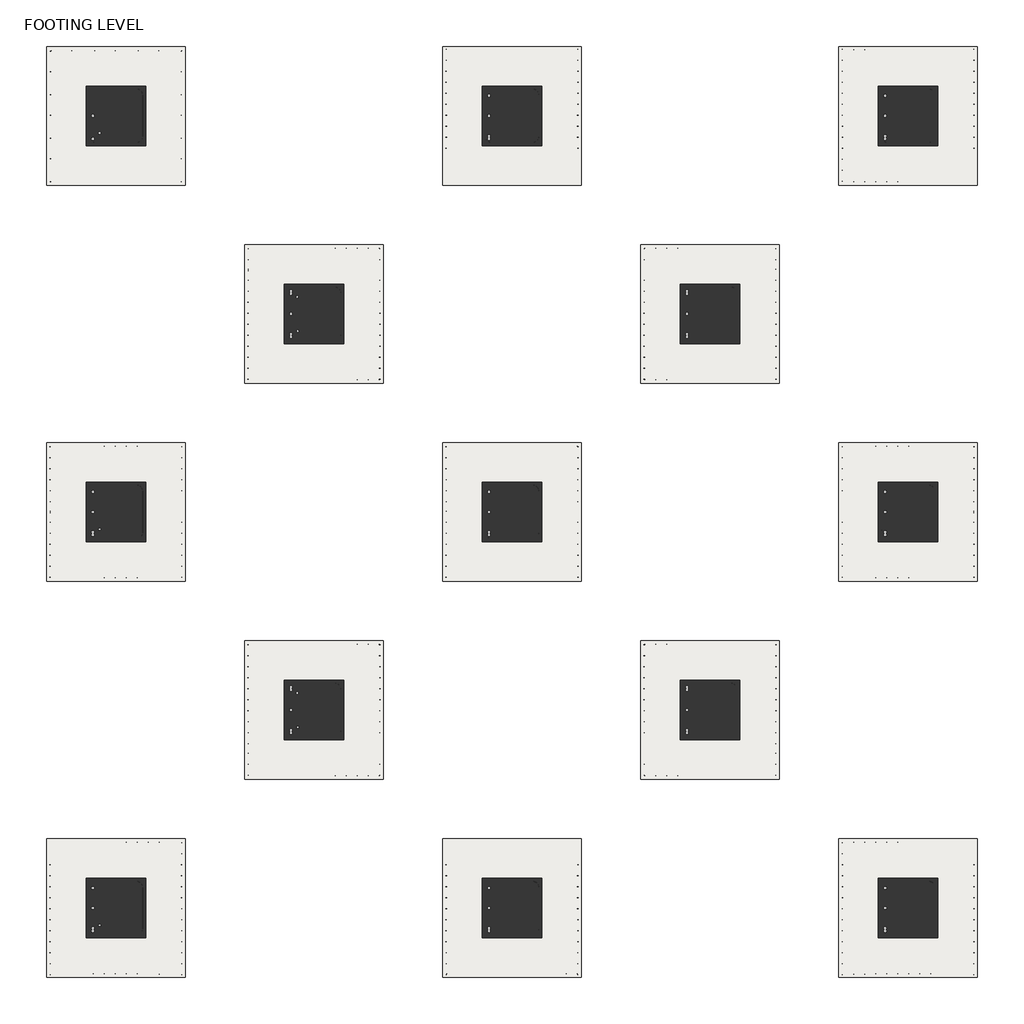
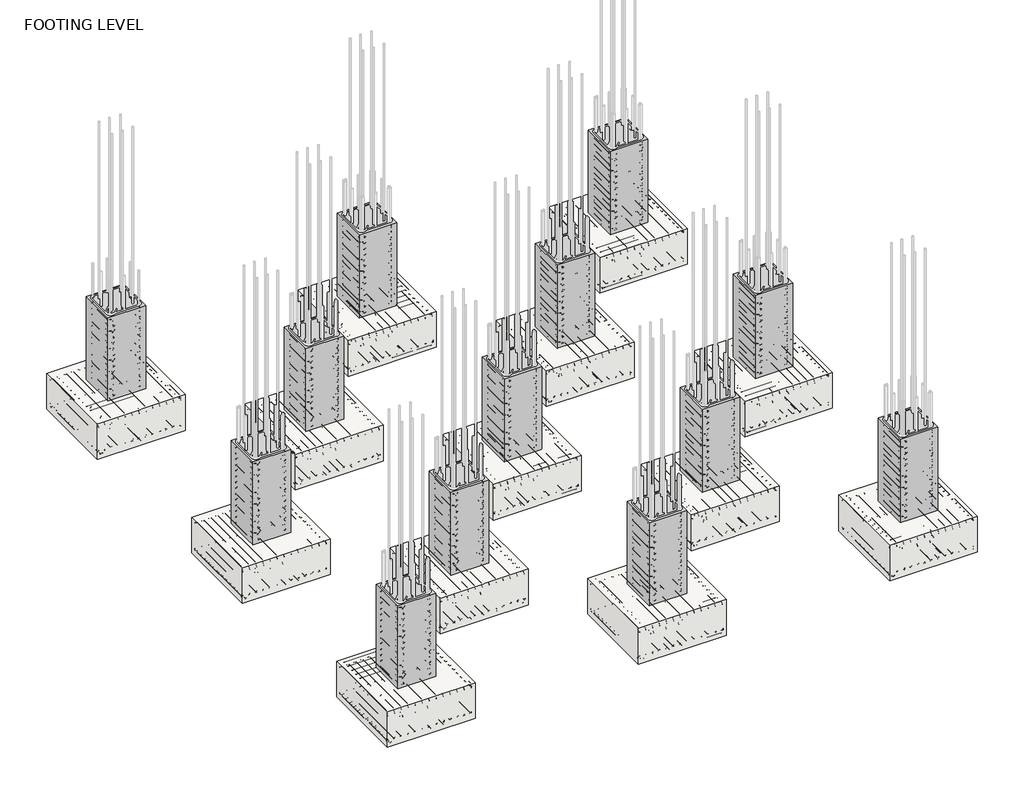
# One storey, part 1 of 10: 13 columns, 13 slabs.
"""IFC4 building model written with IfcOpenShell, lengths in millimetres."""

from ifc_helpers import new_model, si_unit, frame, origin, place, context, project, spatial, polyline, outline, extrude, transform, mapped, element, save
from components import m_footing_rectangular_1800_x_1200_x_450mm_ec84a8aa

model = new_model("IFC4")

# Units and contexts
model_context = context("Model", 3, world=origin())
ifc_project = project(units=[si_unit("LENGTHUNIT", "METRE", prefix="MILLI")], contexts=[model_context])

# Site, building, storey
site = spatial("IfcSite", under=ifc_project)
building = spatial("IfcBuilding", under=site)
storey = spatial("IfcBuildingStorey", under=building, Name="FOOTING LEVEL", Elevation=-2133.6)

# Columns
placement = place(None, origin())
element("IfcColumn", 1, ObjectType="M_Concrete-Rectangular-Column : 3'X3'", at=placement, inside=storey, context=model_context, shape_type="SweptSolid", body=[
    extrude(outline(polyline([(-12383.8269037, 12391.5829396), (-12383.8269037, 11477.1829396), (-13298.2269037, 11477.1829396), (-13298.2269037, 12391.5829396), (-12383.8269037, 12391.5829396)])), frame((0.0, 0.0, -2133.6), z_axis=(0.0, 0.0, 1.0), x_axis=(1.0, 0.0, 0.0)), (0.0, 0.0, 1.0), 2133.6),
])
element("IfcColumn", 2, ObjectType="M_Concrete-Rectangular-Column : 3'X3'", at=placement, inside=storey, context=model_context, shape_type="SweptSolid", body=[
    extrude(outline(polyline([(-12383.8269037, 6295.5829396), (-12383.8269037, 5381.1829396), (-13298.2269037, 5381.1829396), (-13298.2269037, 6295.5829396), (-12383.8269037, 6295.5829396)])), frame((0.0, 0.0, -2133.6), z_axis=(0.0, 0.0, 1.0), x_axis=(1.0, 0.0, 0.0)), (0.0, 0.0, 1.0), 2133.6),
])
element("IfcColumn", 3, ObjectType="M_Concrete-Rectangular-Column : 3'X3'", at=placement, inside=storey, context=model_context, shape_type="SweptSolid", body=[
    extrude(outline(polyline([(-12383.8269037, 199.5829396), (-12383.8269037, -714.8170604), (-13298.2269037, -714.8170604), (-13298.2269037, 199.5829396), (-12383.8269037, 199.5829396)])), frame((0.0, 0.0, -2133.6), z_axis=(0.0, 0.0, 1.0), x_axis=(1.0, 0.0, 0.0)), (0.0, 0.0, 1.0), 2133.6),
])
element("IfcColumn", 4, ObjectType="M_Concrete-Rectangular-Column : 3'X3'", at=placement, inside=storey, context=model_context, shape_type="SweptSolid", body=[
    extrude(outline(polyline([(-9335.8269037, 9343.5829396), (-9335.8269037, 8429.1829396), (-10250.2269037, 8429.1829396), (-10250.2269037, 9343.5829396), (-9335.8269037, 9343.5829396)])), frame((0.0, 0.0, -2133.6), z_axis=(0.0, 0.0, 1.0), x_axis=(1.0, 0.0, 0.0)), (0.0, 0.0, 1.0), 2133.6),
])
element("IfcColumn", 5, ObjectType="M_Concrete-Rectangular-Column : 3'X3'", at=placement, inside=storey, context=model_context, shape_type="SweptSolid", body=[
    extrude(outline(polyline([(-9335.8269037, 3247.5829396), (-9335.8269037, 2333.1829396), (-10250.2269037, 2333.1829396), (-10250.2269037, 3247.5829396), (-9335.8269037, 3247.5829396)])), frame((0.0, 0.0, -2133.6), z_axis=(0.0, 0.0, 1.0), x_axis=(1.0, 0.0, 0.0)), (0.0, 0.0, 1.0), 2133.6),
])
element("IfcColumn", 6, ObjectType="M_Concrete-Rectangular-Column : 3'X3'", at=placement, inside=storey, context=model_context, shape_type="SweptSolid", body=[
    extrude(outline(polyline([(-6287.8269037, 12391.5829396), (-6287.8269037, 11477.1829396), (-7202.2269037, 11477.1829396), (-7202.2269037, 12391.5829396), (-6287.8269037, 12391.5829396)])), frame((0.0, 0.0, -2133.6), z_axis=(0.0, 0.0, 1.0), x_axis=(1.0, 0.0, 0.0)), (0.0, 0.0, 1.0), 2133.6),
])
element("IfcColumn", 7, ObjectType="M_Concrete-Rectangular-Column : 3'X3'", at=placement, inside=storey, context=model_context, shape_type="SweptSolid", body=[
    extrude(outline(polyline([(-6287.8269037, 6295.5829396), (-6287.8269037, 5381.1829396), (-7202.2269037, 5381.1829396), (-7202.2269037, 6295.5829396), (-6287.8269037, 6295.5829396)])), frame((0.0, 0.0, -2133.6), z_axis=(0.0, 0.0, 1.0), x_axis=(1.0, 0.0, 0.0)), (0.0, 0.0, 1.0), 2133.6),
])
element("IfcColumn", 8, ObjectType="M_Concrete-Rectangular-Column : 3'X3'", at=placement, inside=storey, context=model_context, shape_type="SweptSolid", body=[
    extrude(outline(polyline([(-6287.8269037, 199.5829396), (-6287.8269037, -714.8170604), (-7202.2269037, -714.8170604), (-7202.2269037, 199.5829396), (-6287.8269037, 199.5829396)])), frame((0.0, 0.0, -2133.6), z_axis=(0.0, 0.0, 1.0), x_axis=(1.0, 0.0, 0.0)), (0.0, 0.0, 1.0), 2133.6),
])
element("IfcColumn", 9, ObjectType="M_Concrete-Rectangular-Column : 3'X3'", at=placement, inside=storey, context=model_context, shape_type="SweptSolid", body=[
    extrude(outline(polyline([(-3239.8269037, 9343.5829396), (-3239.8269037, 8429.1829396), (-4154.2269037, 8429.1829396), (-4154.2269037, 9343.5829396), (-3239.8269037, 9343.5829396)])), frame((0.0, 0.0, -2133.6), z_axis=(0.0, 0.0, 1.0), x_axis=(1.0, 0.0, 0.0)), (0.0, 0.0, 1.0), 2133.6),
])
element("IfcColumn", 10, ObjectType="M_Concrete-Rectangular-Column : 3'X3'", at=placement, inside=storey, context=model_context, shape_type="SweptSolid", body=[
    extrude(outline(polyline([(-3239.8269037, 3247.5829396), (-3239.8269037, 2333.1829396), (-4154.2269037, 2333.1829396), (-4154.2269037, 3247.5829396), (-3239.8269037, 3247.5829396)])), frame((0.0, 0.0, -2133.6), z_axis=(0.0, 0.0, 1.0), x_axis=(1.0, 0.0, 0.0)), (0.0, 0.0, 1.0), 2133.6),
])
element("IfcColumn", 11, ObjectType="M_Concrete-Rectangular-Column : 3'X3'", at=placement, inside=storey, context=model_context, shape_type="SweptSolid", body=[
    extrude(outline(polyline([(-191.8269037, 12391.5829396), (-191.8269037, 11477.1829396), (-1106.2269037, 11477.1829396), (-1106.2269037, 12391.5829396), (-191.8269037, 12391.5829396)])), frame((0.0, 0.0, -2133.6), z_axis=(0.0, 0.0, 1.0), x_axis=(1.0, 0.0, 0.0)), (0.0, 0.0, 1.0), 2133.6),
])
element("IfcColumn", 12, ObjectType="M_Concrete-Rectangular-Column : 3'X3'", at=placement, inside=storey, context=model_context, shape_type="SweptSolid", body=[
    extrude(outline(polyline([(-191.8269037, 6295.5829396), (-191.8269037, 5381.1829396), (-1106.2269037, 5381.1829396), (-1106.2269037, 6295.5829396), (-191.8269037, 6295.5829396)])), frame((0.0, 0.0, -2133.6), z_axis=(0.0, 0.0, 1.0), x_axis=(1.0, 0.0, 0.0)), (0.0, 0.0, 1.0), 2133.6),
])
element("IfcColumn", 13, ObjectType="M_Concrete-Rectangular-Column : 3'X3'", at=placement, inside=storey, context=model_context, shape_type="SweptSolid", body=[
    extrude(outline(polyline([(-191.8269037, 199.5829396), (-191.8269037, -714.8170604), (-1106.2269037, -714.8170604), (-1106.2269037, 199.5829396), (-191.8269037, 199.5829396)])), frame((0.0, 0.0, -2133.6), z_axis=(0.0, 0.0, 1.0), x_axis=(1.0, 0.0, 0.0)), (0.0, 0.0, 1.0), 2133.6),
])

# Slabs
m_footing_rectangular_1800_x_1200_x_450mm_shape = m_footing_rectangular_1800_x_1200_x_450mm_ec84a8aa(model_context)
element("IfcSlab", 14, ObjectType="M_Footing-Rectangular : 1800 x 1200 x 450mm", at=placement, inside=storey, context=model_context, shape_type="MappedRepresentation", body=[
    mapped(m_footing_rectangular_1800_x_1200_x_450mm_shape, transform((-12841.0269037, 11934.3829396, -2133.6), x_axis=(1.0, 0.0, 0.0), y_axis=(0.0, 1.0, 0.0), z_axis=(0.0, 0.0, 1.0))),
])
element("IfcSlab", 15, ObjectType="M_Footing-Rectangular : 1800 x 1200 x 450mm", at=placement, inside=storey, context=model_context, shape_type="MappedRepresentation", body=[
    mapped(m_footing_rectangular_1800_x_1200_x_450mm_shape, transform((-12841.0269037, 5838.3829396, -2133.6), x_axis=(1.0, 0.0, 0.0), y_axis=(0.0, 1.0, 0.0), z_axis=(0.0, 0.0, 1.0))),
])
element("IfcSlab", 16, ObjectType="M_Footing-Rectangular : 1800 x 1200 x 450mm", at=placement, inside=storey, context=model_context, shape_type="MappedRepresentation", body=[
    mapped(m_footing_rectangular_1800_x_1200_x_450mm_shape, transform((-12841.0269037, -257.6170604, -2133.6), x_axis=(1.0, 0.0, 0.0), y_axis=(0.0, 1.0, 0.0), z_axis=(0.0, 0.0, 1.0))),
])
element("IfcSlab", 17, ObjectType="M_Footing-Rectangular : 1800 x 1200 x 450mm", at=placement, inside=storey, context=model_context, shape_type="MappedRepresentation", body=[
    mapped(m_footing_rectangular_1800_x_1200_x_450mm_shape, transform((-9793.0269037, 8886.3829396, -2133.6), x_axis=(1.0, 0.0, 0.0), y_axis=(0.0, 1.0, 0.0), z_axis=(0.0, 0.0, 1.0))),
])
element("IfcSlab", 18, ObjectType="M_Footing-Rectangular : 1800 x 1200 x 450mm", at=placement, inside=storey, context=model_context, shape_type="MappedRepresentation", body=[
    mapped(m_footing_rectangular_1800_x_1200_x_450mm_shape, transform((-9793.0269037, 2790.3829396, -2133.6), x_axis=(1.0, 0.0, 0.0), y_axis=(0.0, 1.0, 0.0), z_axis=(0.0, 0.0, 1.0))),
])
element("IfcSlab", 19, ObjectType="M_Footing-Rectangular : 1800 x 1200 x 450mm", at=placement, inside=storey, context=model_context, shape_type="MappedRepresentation", body=[
    mapped(m_footing_rectangular_1800_x_1200_x_450mm_shape, transform((-6745.0269037, 11934.3829396, -2133.6), x_axis=(1.0, 0.0, 0.0), y_axis=(0.0, 1.0, 0.0), z_axis=(0.0, 0.0, 1.0))),
])
element("IfcSlab", 20, ObjectType="M_Footing-Rectangular : 1800 x 1200 x 450mm", at=placement, inside=storey, context=model_context, shape_type="MappedRepresentation", body=[
    mapped(m_footing_rectangular_1800_x_1200_x_450mm_shape, transform((-6745.0269037, 5838.3829396, -2133.6), x_axis=(1.0, 0.0, 0.0), y_axis=(0.0, 1.0, 0.0), z_axis=(0.0, 0.0, 1.0))),
])
element("IfcSlab", 21, ObjectType="M_Footing-Rectangular : 1800 x 1200 x 450mm", at=placement, inside=storey, context=model_context, shape_type="MappedRepresentation", body=[
    mapped(m_footing_rectangular_1800_x_1200_x_450mm_shape, transform((-6745.0269037, -257.6170604, -2133.6), x_axis=(1.0, 0.0, 0.0), y_axis=(0.0, 1.0, 0.0), z_axis=(0.0, 0.0, 1.0))),
])
element("IfcSlab", 22, ObjectType="M_Footing-Rectangular : 1800 x 1200 x 450mm", at=placement, inside=storey, context=model_context, shape_type="MappedRepresentation", body=[
    mapped(m_footing_rectangular_1800_x_1200_x_450mm_shape, transform((-3697.0269037, 8886.3829396, -2133.6), x_axis=(1.0, 0.0, 0.0), y_axis=(0.0, 1.0, 0.0), z_axis=(0.0, 0.0, 1.0))),
])
element("IfcSlab", 23, ObjectType="M_Footing-Rectangular : 1800 x 1200 x 450mm", at=placement, inside=storey, context=model_context, shape_type="MappedRepresentation", body=[
    mapped(m_footing_rectangular_1800_x_1200_x_450mm_shape, transform((-3697.0269037, 2790.3829396, -2133.6), x_axis=(1.0, 0.0, 0.0), y_axis=(0.0, 1.0, 0.0), z_axis=(0.0, 0.0, 1.0))),
])
element("IfcSlab", 24, ObjectType="M_Footing-Rectangular : 1800 x 1200 x 450mm", at=placement, inside=storey, context=model_context, shape_type="MappedRepresentation", body=[
    mapped(m_footing_rectangular_1800_x_1200_x_450mm_shape, transform((-649.0269037, 11934.3829396, -2133.6), x_axis=(1.0, 0.0, 0.0), y_axis=(0.0, 1.0, 0.0), z_axis=(0.0, 0.0, 1.0))),
])
element("IfcSlab", 25, ObjectType="M_Footing-Rectangular : 1800 x 1200 x 450mm", at=placement, inside=storey, context=model_context, shape_type="MappedRepresentation", body=[
    mapped(m_footing_rectangular_1800_x_1200_x_450mm_shape, transform((-649.0269037, 5838.3829396, -2133.6), x_axis=(1.0, 0.0, 0.0), y_axis=(0.0, 1.0, 0.0), z_axis=(0.0, 0.0, 1.0))),
])
element("IfcSlab", 26, ObjectType="M_Footing-Rectangular : 1800 x 1200 x 450mm", at=placement, inside=storey, context=model_context, shape_type="MappedRepresentation", body=[
    mapped(m_footing_rectangular_1800_x_1200_x_450mm_shape, transform((-649.0269037, -257.6170604, -2133.6), x_axis=(1.0, 0.0, 0.0), y_axis=(0.0, 1.0, 0.0), z_axis=(0.0, 0.0, 1.0))),
])

save(model, "model.ifc")

# Revit data of these elements
# Grids (mm)
#   "1": line (-12841.027, 14982.383) -> (-12841.027, -1874.247)
#   "2": line (-9793.027, 14982.383) -> (-9793.027, -1874.247)
#   "3": line (-6745.027, 14982.383) -> (-6745.027, -1874.247)
#   "4": line (-3697.027, 14982.383) -> (-3697.027, -1874.247)
#   "5": line (-649.027, 14982.383) -> (-649.027, -1874.247)
#   "6": line (1697.114, 11934.383) -> (-15889.027, 11934.383)
#   "7": line (1697.114, 8886.383) -> (-15889.027, 8886.383)
#   "8": line (1697.114, 5838.383) -> (-15889.027, 5838.383)
#   "9": line (1697.114, 2790.383) -> (-15889.027, 2790.383)
#   "10": line (1697.114, -257.617) -> (-15889.027, -257.617)
# Type "M_Concrete-Rectangular-Column : 3'X3'"
#   b = 3' - 0"
#   h = 3' - 0"
#   Structural Material [instance default] = Concrete, Cast-in-Place gray
# Type "M_Footing-Rectangular : 1800 x 1200 x 450mm"
#   Width = 7' - 0"
#   Length = 7' - 0"
#   Foundation Thickness = 3' - 0"
#   Structural Material [instance default] = Concrete, Cast-in-Place gray
#   Assembly Code = ""
# Elements 1, 2, 3, 4, 5, 6, 7, 8, 9, 10, 11, 12, 13 (IfcColumn, "M_Concrete-Rectangular-Column : 3'X3'")
#   Structural Material = Concrete, Cast-in-Place gray
#   Phase Created = New Construction
#   Materials on its faces: "Concrete, Cast-in-Place gray"
# Elements 14, 15, 16, 17, 18, 19, 20, 21, 22, 23, 24, 25, 26 (IfcSlab, "M_Footing-Rectangular : 1800 x 1200 x 450mm")
#   Structural Material = Concrete, Cast-in-Place gray
#   Phase Created = New Construction
#   Materials on its faces: "Concrete, Cast-in-Place gray"
# Materials
#   "Concrete, Cast-in-Place gray": class "Concrete", colour RGB 192 192 192, transparency 0, Description = "Cast-in-place concrete", Cost = 0
